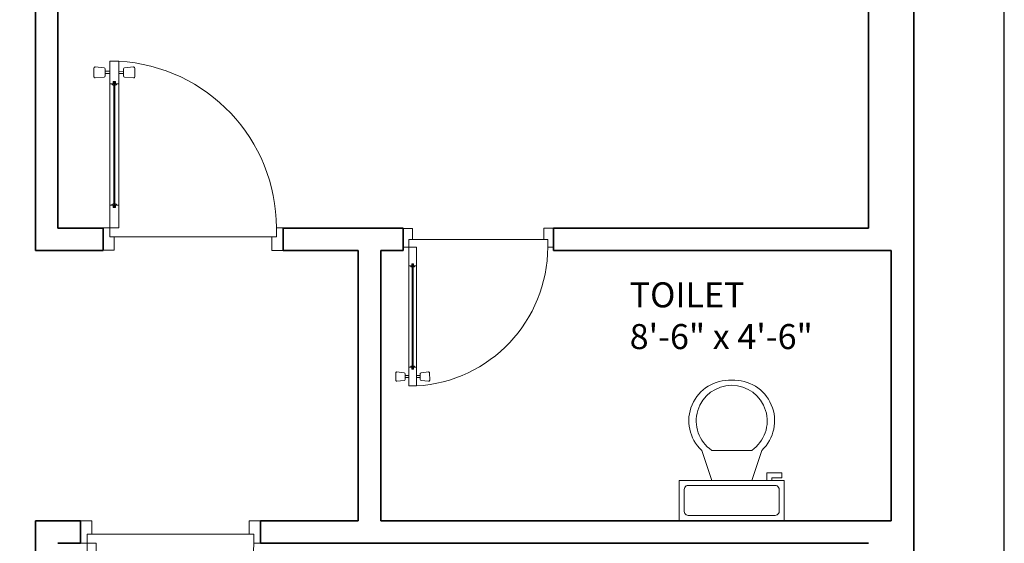
# Model space of a CAD drawing. Units: inches. Extents: x -638 to 186, y -762 to 59.
# Tile 15 of 31: x -168 to 29, y -413 to -308. Entities that reach past the tile are written whole.
import ezdxf

# ---------------------------------------------------------------- set-up
doc = ezdxf.new("R2010")
doc.units = ezdxf.units.IN
for name, color, linetype, lineweight in [('A-ANNO-DIMS', 2, 'Continuous', 18), ('A-AREA-IDEN', 1, 'Continuous', 18), ('A-DOOR', 3, 'Continuous', 18), ('A-FLOR-FIXT', 9, 'Continuous', 18), ('C-PROP', 7, 'Continuous', 25), ('wall', 7, 'Continuous', 35)]:
    doc.layers.add(name, color=color, linetype=linetype, lineweight=lineweight)
doc.styles.get("Standard").update_dxf_attribs({"font": 'arial.ttf'})
doc.dimstyles.new('ISO-25', dxfattribs={"dimtxt": 4, "dimasz": 4, "dimexe": 1.25, "dimexo": 0.625, "dimtad": 0, "dimlunit": 4, "dimtxsty": 'Standard', "dimcen": 2.5, "dimclrt": 256, "dimadec": 0, "dimazin": 0, "dimtfac": 1, "dimtmove": 0, "dimatfit": 3, "dimfxl": 1, "dimfxlon": 1, "dimarcsym": 0})

# ---------------------------------------------------------------- blocks, each defined once
blk = doc.blocks.new('*U4')
for p, q in [((9.5, -6), (9.5, -2)), ((-10, -8.5), (-8, -8.5)), ((-10, -9.5), (-10, -8.5)), ((-7, -9.5), (-10, -9.5)), ((-8, -8.5), (-8, -8)), ((-7, -8), (-7, -9.5)), ((-4, -8), (-6, -14)), ((4, -8), (6, -14)), ((4, -14), (-4, -14))]:
    blk.add_line(p, q)
blk.add_lwpolyline([(10.5, -8), (10.5, 0), (-10.5, 0), (-10.5, -8)], close=True)
for points in [[(8.5, -1), (-8.5, -1)], [(-9.5, -2), (-9.5, -6)], [(-8.5, -7), (8.5, -7)]]:
    blk.add_lwpolyline(points)
for centre, radius, start, end in [((-8.625, -1.875), 0.8839, 81.8699, 188.1301), ((8.625, -1.875), 0.8839, 351.8699, 98.1301), ((-8.625, -6.125), 0.8839, 171.869898, 278.1301), ((8.625, -6.125), 0.8839, 261.8699, 8.1301), ((-0.4772, -19.9188), 8.0953, 133.01722, 273.38), ((0.0374, -19.8731), 7.127, 124.50543, 269.7), ((-0.0373, -19.8731), 7.127, 270.3, 55.4946), ((0.4773, -19.9188), 8.0953, 266.62, 46.9828)]:
    blk.add_arc(centre, radius, start, end)
blk = doc.blocks.new('*D14')
at = {"layer": 'A-ANNO-DIMS', "color": 0, "lineweight": -2, "transparency": 16777216}
for p, q in [((45.41, -42.03), (47.66, -42.03)), ((46.41, -52.03), (46.41, -307.65)), ((46.41, -607.03), (46.41, -351.42)), ((45.41, -617.03), (47.66, -617.03))]:
    blk.add_line(p, q, dxfattribs=at)
at = {"layer": 'A-ANNO-DIMS', "color": 0, "lineweight": 30, "transparency": 16777216}
for points in [[(44.74, -52.03), (48.08, -52.03), (46.41, -42.03)], [(44.74, -607.03), (48.08, -607.03), (46.41, -617.03)]]:
    blk.add_solid(points, dxfattribs=at)
at = {"layer": 'Defpoints', "color": 0, "lineweight": 30, "transparency": 16777216}
for p in [(10.47, -42.03), (10.47, -617.03), (46.41, -617.03)]:
    blk.add_point(p, dxfattribs=at)
at = {"layer": 'A-ANNO-DIMS', "color": 0, "transparency": 16777216, "insert": (46.41, -329.53), "char_height": 10, "attachment_point": 5, "rotation": 90}
blk.add_mtext('47\'-11"', dxfattribs=at)
blk = doc.blocks.new('*D15')
at = {"layer": 'A-ANNO-DIMS', "color": 0, "lineweight": -2, "transparency": 16777216}
for p, q in [((69.33, -24.03), (71.58, -24.03)), ((70.33, -34.03), (70.33, -350.73)), ((70.33, -703.03), (70.33, -386.33)), ((69.33, -713.03), (71.58, -713.03))]:
    blk.add_line(p, q, dxfattribs=at)
at = {"layer": 'A-ANNO-DIMS', "color": 0, "lineweight": 30, "transparency": 16777216}
for points in [[(68.66, -34.03), (72, -34.03), (70.33, -24.03)], [(68.66, -703.03), (72, -703.03), (70.33, -713.03)]]:
    blk.add_solid(points, dxfattribs=at)
at = {"layer": 'Defpoints', "color": 0, "lineweight": 30, "transparency": 16777216}
for p in [(-24.67, -24.03), (-10.56, -713.03), (70.33, -713.03)]:
    blk.add_point(p, dxfattribs=at)
at = {"layer": 'A-ANNO-DIMS', "color": 0, "transparency": 16777216, "insert": (70.33, -368.53), "char_height": 10, "attachment_point": 5, "rotation": 90}
blk.add_mtext('57\'-5"', dxfattribs=at)
blk = doc.blocks.new('DOOR-SWING-36IN')
for p, q in [((35.54, 35.1), (4.05, 35.09)), ((3.16, 4.5), (3.16, 28.79)), ((3.95, 4.05), (3.94, 29.24)), ((4.06, 4.05), (4.06, 29.24)), ((4.18, 4.05), (4.17, 29.24)), ((4.96, 4.5), (4.96, 28.79))]:
    blk.add_line(p, q)
for points in [[(3.16, 33.29), (3.15, 35.09), (4.05, 35.09), (4.05, 37.78), (1.8, 37.78), (1.81, 33.29), (3.16, 33.29)], [(36.44, 33.3), (36.44, 35.1), (35.54, 35.1), (35.54, 37.79), (37.79, 37.8), (37.79, 33.3), (36.44, 33.3)], [(4.28, 28.79), (4.96, 28.79), (4.95, 33.29), (3.16, 33.29), (3.16, 28.79), (3.83, 28.79), (3.83, 29.24), (4.28, 29.24), (4.28, 28.79)], [(4.29, 4.5), (4.96, 4.5), (4.96, 0), (3.17, 0), (3.16, 4.5), (3.84, 4.5), (3.84, 4.05), (4.29, 4.05), (4.29, 4.5)]]:
    blk.add_lwpolyline(points)
for points in [[(2.05, 3.17), (0.25, 3.35, 0.443716), (0, 3.12), (0, 1.37, 0.443716), (0.25, 1.15), (2.05, 1.33, 0.385314), (2.25, 1.55), (2.25, 2.94, 0.385314)], [(6.08, 3.17), (7.88, 3.35, -0.443716), (8.13, 3.13), (8.13, 1.37, -0.443716), (7.88, 1.15), (6.08, 1.33, -0.385314), (5.88, 1.55), (5.88, 2.95, -0.385314)]]:
    blk.add_lwpolyline(points, format="xyb", close=True)
for points in [[(3.16, 2.47), (2.25, 2.47), (2.25, 2.02), (3.17, 2.02)], [(4.96, 2.47), (5.88, 2.47), (5.88, 2.03), (4.96, 2.02)]]:
    blk.add_lwpolyline(points, close=True)
for centre, radius, start, end in [((3.06, 33.32), 33.38, 273.2653, 359.953), ((3.92, 28.83), 0.371, 186.4522, 273.3078), ((4.19, 28.83), 0.371, 266.7282, 353.5838), ((3.93, 4.46), 0.371, 86.7282, 173.5838), ((4.2, 4.46), 0.371, 6.4522, 93.3078)]:
    blk.add_arc(centre, radius, start, end)
blk = doc.blocks.new('DOOR-SWING-30IN')
for p, q in [((29.62, 29.25), (3.38, 29.24)), ((2.64, 3.75), (2.63, 23.99)), ((3.29, 3.37), (3.29, 24.37)), ((3.39, 3.37), (3.38, 24.37)), ((3.48, 3.37), (3.47, 24.37)), ((4.14, 3.75), (4.13, 23.99))]:
    blk.add_line(p, q)
for points in [[(2.63, 27.74), (2.63, 29.24), (3.38, 29.24), (3.38, 31.49), (1.5, 31.49), (1.51, 27.74), (2.63, 27.74)], [(30.37, 27.75), (30.37, 29.25), (29.62, 29.25), (29.62, 31.5), (31.5, 31.5), (31.5, 27.75), (30.37, 27.75)], [(3.57, 23.99), (4.13, 23.99), (4.13, 27.74), (2.63, 27.74), (2.63, 23.99), (3.19, 23.99), (3.19, 24.37), (3.57, 24.37), (3.57, 23.99)], [(3.57, 3.75), (4.14, 3.75), (4.14, 0), (2.64, 0), (2.64, 3.75), (3.2, 3.75), (3.2, 3.37), (3.57, 3.37), (3.57, 3.75)]]:
    blk.add_lwpolyline(points)
for points in [[(1.71, 2.64), (0.21, 2.79, 0.443716), (0, 2.6), (0, 1.14, 0.443716), (0.21, 0.96), (1.71, 1.11, 0.385314), (1.87, 1.29), (1.87, 2.45, 0.385314)], [(5.07, 2.64), (6.57, 2.79, -0.443716), (6.77, 2.61), (6.78, 1.15, -0.443716), (6.57, 0.96), (5.07, 1.11, -0.385314), (4.9, 1.3), (4.9, 2.46, -0.385314)]]:
    blk.add_lwpolyline(points, format="xyb", close=True)
for points in [[(2.64, 2.06), (1.87, 2.06), (1.87, 1.69), (2.64, 1.69)], [(4.14, 2.06), (4.9, 2.06), (4.9, 1.69), (4.14, 1.69)]]:
    blk.add_lwpolyline(points, close=True)
for centre, radius, start, end in [((2.55, 27.77), 27.82, 273.2653, 359.953), ((3.27, 24.03), 0.309, 186.4522, 273.3078), ((3.49, 24.03), 0.309, 266.7282, 353.5838), ((3.28, 3.71), 0.309, 86.7282, 173.5838), ((3.5, 3.71), 0.309, 6.4522, 93.3078)]:
    blk.add_arc(centre, radius, start, end)
blk = doc.blocks.new('*D38')
at = {"layer": 'A-ANNO-DIMS', "color": 0, "lineweight": -2, "transparency": 16777216}
for p, q in [((182.66, -280.53), (184.91, -280.53)), ((183.66, -284.53), (183.66, -371.73)), ((183.66, -473.53), (183.66, -386.34)), ((182.66, -477.53), (184.91, -477.53))]:
    blk.add_line(p, q, dxfattribs=at)
at = {"layer": 'A-ANNO-DIMS', "color": 0, "lineweight": 30, "transparency": 16777216}
for points in [[(183, -284.53), (184.33, -284.53), (183.66, -280.53)], [(183, -473.53), (184.33, -473.53), (183.66, -477.53)]]:
    blk.add_solid(points, dxfattribs=at)
at = {"layer": 'Defpoints', "color": 0, "lineweight": 30, "transparency": 16777216}
for p in [(-404.53, -280.53), (-404.53, -477.53), (183.66, -477.53)]:
    blk.add_point(p, dxfattribs=at)
at = {"layer": 'A-ANNO-DIMS', "transparency": 16777216, "insert": (183.66, -379.03), "char_height": 4, "attachment_point": 5, "rotation": 90}
blk.add_mtext('16\'-5"', dxfattribs=at)
blk = doc.blocks.new('*D56')
at = {"layer": 'A-ANNO-DIMS', "color": 0, "lineweight": -2, "transparency": 16777216}
for p, q in [((-165.03, 52.02), (-165.03, 54.27)), ((-100.53, 52.02), (-100.53, 54.27)), ((-161.03, 53.02), (-143.38, 53.02)), ((-104.53, 53.02), (-122.17, 53.02))]:
    blk.add_line(p, q, dxfattribs=at)
at = {"layer": 'A-ANNO-DIMS', "color": 0, "lineweight": 30, "transparency": 16777216}
for points in [[(-161.03, 53.68), (-161.03, 52.35), (-165.03, 53.02)], [(-104.53, 53.68), (-104.53, 52.35), (-100.53, 53.02)]]:
    blk.add_solid(points, dxfattribs=at)
at = {"layer": 'Defpoints', "color": 0, "lineweight": 30, "transparency": 16777216}
for p in [(-100.53, 53.02), (-165.03, -408.03), (-100.53, -408.03)]:
    blk.add_point(p, dxfattribs=at)
at = {"layer": 'A-ANNO-DIMS', "transparency": 16777216, "insert": (-132.78, 53.02), "char_height": 4, "attachment_point": 5}
blk.add_mtext('5\'-4 1/2"', dxfattribs=at)

msp = doc.modelspace()

# ---------------------------------------------------------------- linework, layer by layer
at = {"layer": 'C-PROP'}
msp.add_line((28.474, -24.033), (28.474, -713.033), dxfattribs=at)
at = {"layer": 'wall'}
for p, q in [((10.474, -42.033), (10.474, -617.033)), ((-165.026, -197.592), (-165.026, -354.033)), ((-160.526, -205.533), (-160.526, -349.533)), ((1.474, -205.533), (1.474, -349.533)), ((-160.526, -349.533), (-151.526, -349.533)), ((-151.526, -349.533), (-151.526, -354.033)), ((-115.526, -349.533), (-115.526, -354.033)), ((-115.526, -349.533), (-91.526, -349.533)), ((-91.526, -354.033), (-91.526, -349.533)), ((-61.526, -354.033), (-61.526, -349.533)), ((-61.526, -349.533), (1.474, -349.533)), ((-160.526, -354.033), (-165.026, -354.033)), ((-160.526, -354.033), (-151.526, -354.033)), ((-115.526, -354.033), (-105.026, -354.033)), ((-105.026, -354.033), (-100.526, -354.033)), ((-100.526, -354.033), (-100.526, -408.033)), ((-96.026, -354.033), (-91.526, -354.033)), ((-96.026, -354.033), (-96.026, -408.033)), ((-61.526, -354.033), (5.974, -354.033)), ((5.974, -354.033), (5.974, -408.033)), ((-160.526, -408.033), (-165.026, -408.033)), ((-165.026, -408.033), (-165.026, -539.033)), ((-160.526, -408.033), (-156.026, -408.033)), ((-156.026, -408.033), (-156.026, -412.533)), ((-120.026, -408.033), (-120.026, -412.533)), ((-120.026, -408.033), (-100.526, -408.033)), ((-96.026, -408.033), (5.974, -408.033)), ((-160.526, -412.533), (-156.026, -412.533)), ((-120.026, -412.533), (1.474, -412.533))]:
    msp.add_line(p, q, dxfattribs=at)

# ---------------------------------------------------------------- block references
at = {"layer": 'A-DOOR', "extrusion": (0, 0, -1), "zscale": -1, "rotation": 180}
msp.add_blockref('DOOR-SWING-36IN', (153.329, -316.206), dxfattribs=at)
at = {"layer": 'A-DOOR'}
for name, p in [('DOOR-SWING-30IN', (-93.03, -381.089)), ('DOOR-SWING-36IN', (-157.83, -445.817))]:
    msp.add_blockref(name, p, dxfattribs=at)
at = {"layer": 'A-FLOR-FIXT', "rotation": 180}
msp.add_blockref('*U4', (-25.894, -407.956), dxfattribs=at)

# ---------------------------------------------------------------- texts
at = {"layer": 'A-AREA-IDEN', "insert": (-46.285, -360.391), "char_height": 5, "attachment_point": 1}
msp.add_mtext_dynamic_manual_height_columns('\\A1;{TOILET\\P8\'-6" x 4\'-6"}', width=99.04816, gutter_width=12.5, heights=[0], dxfattribs=at)

# ---------------------------------------------------------------- dimensions: what is measured, and where the dimension line sits
at = {"layer": 'A-ANNO-DIMS'}
dim = msp.add_linear_dim(base=(-100.526, 53.017), p1=(-165.026, -408.033), p2=(-100.526, -408.033), dimstyle='ISO-25', override={"dimdec": 1, "dimlfac": 1, "dimrnd": 0, "dimzin": 1, "dimdsep": 46, "dimlunit": 4, "dimfrac": 2}, dxfattribs=at)
dim.commit()
dim.dimension.update_dxf_attribs({"geometry": '*D56', "text_midpoint": (-132.776, 53.017)})
for base, p1, p2, override, picture, middle in [((70.331, -713.033), (-24.669, -24.033), (-10.563, -713.033), {"dimtxt": 10, "dimasz": 10, "dimclrd": 0, "dimclre": 0, "dimclrt": 0}, '*D15', (70.331, -368.533)), ((46.411, -617.033), (10.474, -42.033), (10.474, -617.033), {"dimtxt": 10, "dimasz": 10, "dimclrd": 0, "dimclre": 0, "dimclrt": 0}, '*D14', (46.411, -329.533)), ((183.663, -477.533), (-404.526, -280.533), (-404.526, -477.533), {"dimdec": 1, "dimlfac": 1, "dimrnd": 0, "dimzin": 1, "dimdsep": 46, "dimlunit": 4, "dimfrac": 2}, '*D38', (183.663, -379.033))]:
    dim = msp.add_linear_dim(base=base, p1=p1, p2=p2, angle=90, dimstyle='ISO-25', override=override, dxfattribs=at)
    dim.commit()
    dim.dimension.update_dxf_attribs({"geometry": picture, "text_midpoint": middle})

doc.saveas('drawing.dxf')
